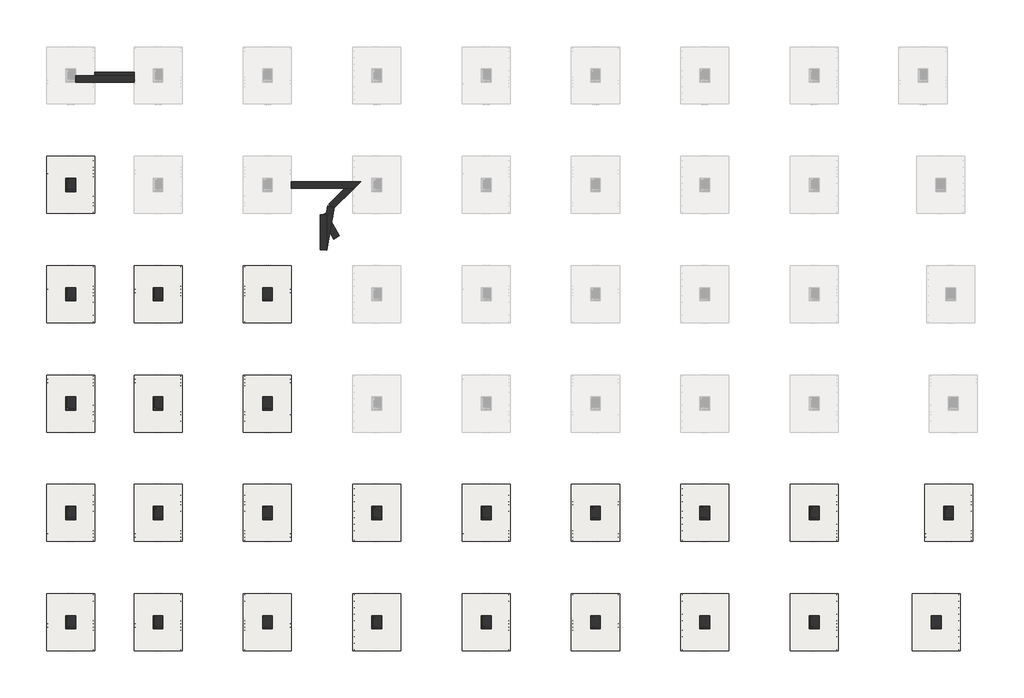
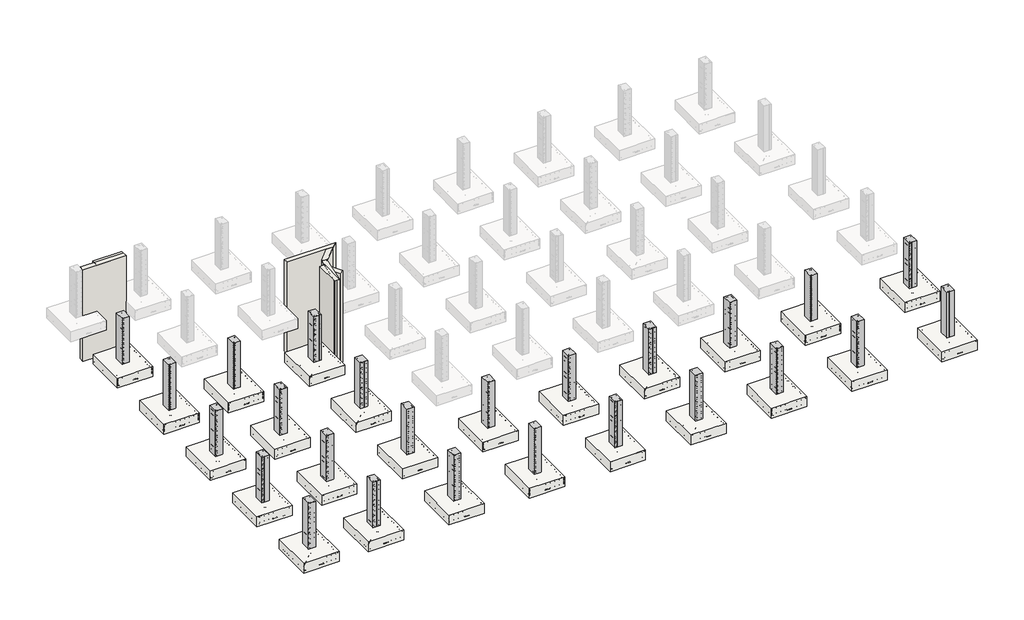
# One storey, part 1 of 33: 25 columns, 25 slabs, 9 walls.
"""IFC4 building model written with IfcOpenShell, lengths in millimetres."""

from ifc_helpers import new_model, si_unit, frame, origin, place, context, project, spatial, polyline, outline, extrude, faceted_brep, element, save

model = new_model("IFC4")

# Units and contexts
model_context = context("Model", 3, world=origin())
ifc_project = project(units=[si_unit("LENGTHUNIT", "METRE", prefix="MILLI")], contexts=[model_context])

# Site, building, storey
site = spatial("IfcSite", under=ifc_project)
building = spatial("IfcBuilding", under=site)
storey = spatial("IfcBuildingStorey", under=building, Elevation=-3000.0)

# Columns
placement = place(None, origin())
element("IfcColumn", 1, ObjectType="M_Concrete-Rectangular-Column : 300 x 450mm", at=placement, inside=storey, context=model_context, shape_type="SweptSolid", body=[
    extrude(outline(polyline([(-13414.8142742, 12007.0891866), (-13414.8142742, 11397.4891866), (-13864.8142742, 11397.4891866), (-13864.8142742, 12007.0891866), (-13414.8142742, 12007.0891866)])), frame((0.0, 0.0, -3000.0), z_axis=(0.0, 0.0, 1.0), x_axis=(1.0, 0.0, 0.0)), (0.0, 0.0, 1.0), 3000.0),
])
element("IfcColumn", 2, ObjectType="M_Concrete-Rectangular-Column : 300 x 450mm", at=placement, inside=storey, context=model_context, shape_type="SweptSolid", body=[
    extrude(outline(polyline([(-13414.8142742, 7007.0891866), (-13414.8142742, 6397.4891866), (-13864.8142742, 6397.4891866), (-13864.8142742, 7007.0891866), (-13414.8142742, 7007.0891866)])), frame((0.0, 0.0, -3000.0), z_axis=(0.0, 0.0, 1.0), x_axis=(1.0, 0.0, 0.0)), (0.0, 0.0, 1.0), 3000.0),
])
element("IfcColumn", 3, ObjectType="M_Concrete-Rectangular-Column : 300 x 450mm", at=placement, inside=storey, context=model_context, shape_type="SweptSolid", body=[
    extrude(outline(polyline([(-13414.8142742, 2007.0891866), (-13414.8142742, 1397.4891866), (-13864.8142742, 1397.4891866), (-13864.8142742, 2007.0891866), (-13414.8142742, 2007.0891866)])), frame((0.0, 0.0, -3000.0), z_axis=(0.0, 0.0, 1.0), x_axis=(1.0, 0.0, 0.0)), (0.0, 0.0, 1.0), 3000.0),
])
element("IfcColumn", 4, ObjectType="M_Concrete-Rectangular-Column : 300 x 450mm", at=placement, inside=storey, context=model_context, shape_type="SweptSolid", body=[
    extrude(outline(polyline([(-13414.8142742, -2992.9108134), (-13414.8142742, -3602.5108134), (-13864.8142742, -3602.5108134), (-13864.8142742, -2992.9108134), (-13414.8142742, -2992.9108134)])), frame((0.0, 0.0, -3000.0), z_axis=(0.0, 0.0, 1.0), x_axis=(1.0, 0.0, 0.0)), (0.0, 0.0, 1.0), 3000.0),
])
element("IfcColumn", 5, ObjectType="M_Concrete-Rectangular-Column : 300 x 450mm", at=placement, inside=storey, context=model_context, shape_type="SweptSolid", body=[
    extrude(outline(polyline([(-13414.8142742, -7992.9108134), (-13414.8142742, -8602.5108134), (-13864.8142742, -8602.5108134), (-13864.8142742, -7992.9108134), (-13414.8142742, -7992.9108134)])), frame((0.0, 0.0, -3000.0), z_axis=(0.0, 0.0, 1.0), x_axis=(1.0, 0.0, 0.0)), (0.0, 0.0, 1.0), 3000.0),
])
element("IfcColumn", 6, ObjectType="M_Concrete-Rectangular-Column : 300 x 450mm", at=placement, inside=storey, context=model_context, shape_type="SweptSolid", body=[
    extrude(outline(polyline([(-9414.8142742, 7007.0891866), (-9414.8142742, 6397.4891866), (-9864.8142742, 6397.4891866), (-9864.8142742, 7007.0891866), (-9414.8142742, 7007.0891866)])), frame((0.0, 0.0, -3000.0), z_axis=(0.0, 0.0, 1.0), x_axis=(1.0, 0.0, 0.0)), (0.0, 0.0, 1.0), 3000.0),
])
element("IfcColumn", 7, ObjectType="M_Concrete-Rectangular-Column : 300 x 450mm", at=placement, inside=storey, context=model_context, shape_type="SweptSolid", body=[
    extrude(outline(polyline([(-9414.8142742, 2007.0891866), (-9414.8142742, 1397.4891866), (-9864.8142742, 1397.4891866), (-9864.8142742, 2007.0891866), (-9414.8142742, 2007.0891866)])), frame((0.0, 0.0, -3000.0), z_axis=(0.0, 0.0, 1.0), x_axis=(1.0, 0.0, 0.0)), (0.0, 0.0, 1.0), 3000.0),
])
element("IfcColumn", 8, ObjectType="M_Concrete-Rectangular-Column : 300 x 450mm", at=placement, inside=storey, context=model_context, shape_type="SweptSolid", body=[
    extrude(outline(polyline([(-9414.8142742, -2992.9108134), (-9414.8142742, -3602.5108134), (-9864.8142742, -3602.5108134), (-9864.8142742, -2992.9108134), (-9414.8142742, -2992.9108134)])), frame((0.0, 0.0, -3000.0), z_axis=(0.0, 0.0, 1.0), x_axis=(1.0, 0.0, 0.0)), (0.0, 0.0, 1.0), 3000.0),
])
element("IfcColumn", 9, ObjectType="M_Concrete-Rectangular-Column : 300 x 450mm", at=placement, inside=storey, context=model_context, shape_type="SweptSolid", body=[
    extrude(outline(polyline([(-9414.8142742, -7992.9108134), (-9414.8142742, -8602.5108134), (-9864.8142742, -8602.5108134), (-9864.8142742, -7992.9108134), (-9414.8142742, -7992.9108134)])), frame((0.0, 0.0, -3000.0), z_axis=(0.0, 0.0, 1.0), x_axis=(1.0, 0.0, 0.0)), (0.0, 0.0, 1.0), 3000.0),
])
element("IfcColumn", 10, ObjectType="M_Concrete-Rectangular-Column : 300 x 450mm", at=placement, inside=storey, context=model_context, shape_type="SweptSolid", body=[
    extrude(outline(polyline([(-4414.8142742, 7007.0891866), (-4414.8142742, 6397.4891866), (-4864.8142742, 6397.4891866), (-4864.8142742, 7007.0891866), (-4414.8142742, 7007.0891866)])), frame((0.0, 0.0, -3000.0), z_axis=(0.0, 0.0, 1.0), x_axis=(1.0, 0.0, 0.0)), (0.0, 0.0, 1.0), 3000.0),
])
element("IfcColumn", 11, ObjectType="M_Concrete-Rectangular-Column : 300 x 450mm", at=placement, inside=storey, context=model_context, shape_type="SweptSolid", body=[
    extrude(outline(polyline([(-4414.8142742, 2007.0891866), (-4414.8142742, 1397.4891866), (-4864.8142742, 1397.4891866), (-4864.8142742, 2007.0891866), (-4414.8142742, 2007.0891866)])), frame((0.0, 0.0, -3000.0), z_axis=(0.0, 0.0, 1.0), x_axis=(1.0, 0.0, 0.0)), (0.0, 0.0, 1.0), 3000.0),
])
element("IfcColumn", 12, ObjectType="M_Concrete-Rectangular-Column : 300 x 450mm", at=placement, inside=storey, context=model_context, shape_type="SweptSolid", body=[
    extrude(outline(polyline([(-4414.8142742, -2992.9108134), (-4414.8142742, -3602.5108134), (-4864.8142742, -3602.5108134), (-4864.8142742, -2992.9108134), (-4414.8142742, -2992.9108134)])), frame((0.0, 0.0, -3000.0), z_axis=(0.0, 0.0, 1.0), x_axis=(1.0, 0.0, 0.0)), (0.0, 0.0, 1.0), 3000.0),
])
element("IfcColumn", 13, ObjectType="M_Concrete-Rectangular-Column : 300 x 450mm", at=placement, inside=storey, context=model_context, shape_type="SweptSolid", body=[
    extrude(outline(polyline([(-4414.8142742, -7992.9108134), (-4414.8142742, -8602.5108134), (-4864.8142742, -8602.5108134), (-4864.8142742, -7992.9108134), (-4414.8142742, -7992.9108134)])), frame((0.0, 0.0, -3000.0), z_axis=(0.0, 0.0, 1.0), x_axis=(1.0, 0.0, 0.0)), (0.0, 0.0, 1.0), 3000.0),
])
element("IfcColumn", 14, ObjectType="M_Concrete-Rectangular-Column : 300 x 450mm", at=placement, inside=storey, context=model_context, shape_type="SweptSolid", body=[
    extrude(outline(polyline([(585.1857258, -2992.9108134), (585.1857258, -3602.5108134), (135.1857258, -3602.5108134), (135.1857258, -2992.9108134), (585.1857258, -2992.9108134)])), frame((0.0, 0.0, -3000.0), z_axis=(0.0, 0.0, 1.0), x_axis=(1.0, 0.0, 0.0)), (0.0, 0.0, 1.0), 3000.0),
])
element("IfcColumn", 15, ObjectType="M_Concrete-Rectangular-Column : 300 x 450mm", at=placement, inside=storey, context=model_context, shape_type="SweptSolid", body=[
    extrude(outline(polyline([(585.1857258, -7992.9108134), (585.1857258, -8602.5108134), (135.1857258, -8602.5108134), (135.1857258, -7992.9108134), (585.1857258, -7992.9108134)])), frame((0.0, 0.0, -3000.0), z_axis=(0.0, 0.0, 1.0), x_axis=(1.0, 0.0, 0.0)), (0.0, 0.0, 1.0), 3000.0),
])
element("IfcColumn", 16, ObjectType="M_Concrete-Rectangular-Column : 300 x 450mm", at=placement, inside=storey, context=model_context, shape_type="SweptSolid", body=[
    extrude(outline(polyline([(5585.1857258, -2992.9108134), (5585.1857258, -3602.5108134), (5135.1857258, -3602.5108134), (5135.1857258, -2992.9108134), (5585.1857258, -2992.9108134)])), frame((0.0, 0.0, -3000.0), z_axis=(0.0, 0.0, 1.0), x_axis=(1.0, 0.0, 0.0)), (0.0, 0.0, 1.0), 3000.0),
])
element("IfcColumn", 17, ObjectType="M_Concrete-Rectangular-Column : 300 x 450mm", at=placement, inside=storey, context=model_context, shape_type="SweptSolid", body=[
    extrude(outline(polyline([(5585.1857258, -7992.9108134), (5585.1857258, -8602.5108134), (5135.1857258, -8602.5108134), (5135.1857258, -7992.9108134), (5585.1857258, -7992.9108134)])), frame((0.0, 0.0, -3000.0), z_axis=(0.0, 0.0, 1.0), x_axis=(1.0, 0.0, 0.0)), (0.0, 0.0, 1.0), 3000.0),
])
element("IfcColumn", 18, ObjectType="M_Concrete-Rectangular-Column : 300 x 450mm", at=placement, inside=storey, context=model_context, shape_type="SweptSolid", body=[
    extrude(outline(polyline([(10585.1857258, -2992.9108134), (10585.1857258, -3602.5108134), (10135.1857258, -3602.5108134), (10135.1857258, -2992.9108134), (10585.1857258, -2992.9108134)])), frame((0.0, 0.0, -3000.0), z_axis=(0.0, 0.0, 1.0), x_axis=(1.0, 0.0, 0.0)), (0.0, 0.0, 1.0), 3000.0),
])
element("IfcColumn", 19, ObjectType="M_Concrete-Rectangular-Column : 300 x 450mm", at=placement, inside=storey, context=model_context, shape_type="SweptSolid", body=[
    extrude(outline(polyline([(10585.1857258, -7992.9108134), (10585.1857258, -8602.5108134), (10135.1857258, -8602.5108134), (10135.1857258, -7992.9108134), (10585.1857258, -7992.9108134)])), frame((0.0, 0.0, -3000.0), z_axis=(0.0, 0.0, 1.0), x_axis=(1.0, 0.0, 0.0)), (0.0, 0.0, 1.0), 3000.0),
])
element("IfcColumn", 20, ObjectType="M_Concrete-Rectangular-Column : 300 x 450mm", at=placement, inside=storey, context=model_context, shape_type="SweptSolid", body=[
    extrude(outline(polyline([(15585.1857258, -2992.9108134), (15585.1857258, -3602.5108134), (15135.1857258, -3602.5108134), (15135.1857258, -2992.9108134), (15585.1857258, -2992.9108134)])), frame((0.0, 0.0, -3000.0), z_axis=(0.0, 0.0, 1.0), x_axis=(1.0, 0.0, 0.0)), (0.0, 0.0, 1.0), 3000.0),
])
element("IfcColumn", 21, ObjectType="M_Concrete-Rectangular-Column : 300 x 450mm", at=placement, inside=storey, context=model_context, shape_type="SweptSolid", body=[
    extrude(outline(polyline([(15585.1857258, -7992.9108134), (15585.1857258, -8602.5108134), (15135.1857258, -8602.5108134), (15135.1857258, -7992.9108134), (15585.1857258, -7992.9108134)])), frame((0.0, 0.0, -3000.0), z_axis=(0.0, 0.0, 1.0), x_axis=(1.0, 0.0, 0.0)), (0.0, 0.0, 1.0), 3000.0),
])
element("IfcColumn", 22, ObjectType="M_Concrete-Rectangular-Column : 300 x 450mm", at=placement, inside=storey, context=model_context, shape_type="SweptSolid", body=[
    extrude(outline(polyline([(20585.1857258, -2992.9108134), (20585.1857258, -3602.5108134), (20135.1857258, -3602.5108134), (20135.1857258, -2992.9108134), (20585.1857258, -2992.9108134)])), frame((0.0, 0.0, -3000.0), z_axis=(0.0, 0.0, 1.0), x_axis=(1.0, 0.0, 0.0)), (0.0, 0.0, 1.0), 3000.0),
])
element("IfcColumn", 23, ObjectType="M_Concrete-Rectangular-Column : 300 x 450mm", at=placement, inside=storey, context=model_context, shape_type="SweptSolid", body=[
    extrude(outline(polyline([(20585.1857258, -7992.9108134), (20585.1857258, -8602.5108134), (20135.1857258, -8602.5108134), (20135.1857258, -7992.9108134), (20585.1857258, -7992.9108134)])), frame((0.0, 0.0, -3000.0), z_axis=(0.0, 0.0, 1.0), x_axis=(1.0, 0.0, 0.0)), (0.0, 0.0, 1.0), 3000.0),
])
element("IfcColumn", 24, ObjectType="M_Concrete-Rectangular-Column : 300 x 450mm", at=placement, inside=storey, context=model_context, shape_type="SweptSolid", body=[
    extrude(outline(polyline([(26731.4237106, -2992.9108134), (26731.4237106, -3602.5108134), (26281.4237106, -3602.5108134), (26281.4237106, -2992.9108134), (26731.4237106, -2992.9108134)])), frame((0.0, 0.0, -3000.0), z_axis=(0.0, 0.0, 1.0), x_axis=(1.0, 0.0, 0.0)), (0.0, 0.0, 1.0), 3000.0),
])
element("IfcColumn", 25, ObjectType="M_Concrete-Rectangular-Column : 300 x 450mm", at=placement, inside=storey, context=model_context, shape_type="SweptSolid", body=[
    extrude(outline(polyline([(26167.6833949, -7992.9108134), (26167.6833949, -8602.5108134), (25717.6833949, -8602.5108134), (25717.6833949, -7992.9108134), (26167.6833949, -7992.9108134)])), frame((0.0, 0.0, -3000.0), z_axis=(0.0, 0.0, 1.0), x_axis=(1.0, 0.0, 0.0)), (0.0, 0.0, 1.0), 3000.0),
])

# Slabs
element("IfcSlab", 26, ObjectType="M_Footing-Rectangular : 650X2200X2600", at=placement, inside=storey, context=model_context, shape_type="SweptSolid", body=[
    extrude(outline(polyline([(-12539.8142742, 13002.2891866), (-12539.8142742, 10402.2891866), (-14739.8142742, 10402.2891866), (-14739.8142742, 13002.2891866), (-12539.8142742, 13002.2891866)])), frame((0.0, 0.0, -3650.0), z_axis=(0.0, 0.0, 1.0), x_axis=(1.0, 0.0, 0.0)), (0.0, 0.0, 1.0), 650.0),
])
element("IfcSlab", 27, ObjectType="M_Footing-Rectangular : 650X2200X2600", at=placement, inside=storey, context=model_context, shape_type="SweptSolid", body=[
    extrude(outline(polyline([(-12539.8142742, 8002.2891866), (-12539.8142742, 5402.2891866), (-14739.8142742, 5402.2891866), (-14739.8142742, 8002.2891866), (-12539.8142742, 8002.2891866)])), frame((0.0, 0.0, -3650.0), z_axis=(0.0, 0.0, 1.0), x_axis=(1.0, 0.0, 0.0)), (0.0, 0.0, 1.0), 650.0),
])
element("IfcSlab", 28, ObjectType="M_Footing-Rectangular : 650X2200X2600", at=placement, inside=storey, context=model_context, shape_type="SweptSolid", body=[
    extrude(outline(polyline([(-12539.8142742, 3002.2891866), (-12539.8142742, 402.2891866), (-14739.8142742, 402.2891866), (-14739.8142742, 3002.2891866), (-12539.8142742, 3002.2891866)])), frame((0.0, 0.0, -3650.0), z_axis=(0.0, 0.0, 1.0), x_axis=(1.0, 0.0, 0.0)), (0.0, 0.0, 1.0), 650.0),
])
element("IfcSlab", 29, ObjectType="M_Footing-Rectangular : 650X2200X2600", at=placement, inside=storey, context=model_context, shape_type="SweptSolid", body=[
    extrude(outline(polyline([(-12539.8142742, -1997.7108134), (-12539.8142742, -4597.7108134), (-14739.8142742, -4597.7108134), (-14739.8142742, -1997.7108134), (-12539.8142742, -1997.7108134)])), frame((0.0, 0.0, -3650.0), z_axis=(0.0, 0.0, 1.0), x_axis=(1.0, 0.0, 0.0)), (0.0, 0.0, 1.0), 650.0),
])
element("IfcSlab", 30, ObjectType="M_Footing-Rectangular : 650X2200X2600", at=placement, inside=storey, context=model_context, shape_type="SweptSolid", body=[
    extrude(outline(polyline([(-12539.8142742, -6997.7108134), (-12539.8142742, -9597.7108134), (-14739.8142742, -9597.7108134), (-14739.8142742, -6997.7108134), (-12539.8142742, -6997.7108134)])), frame((0.0, 0.0, -3650.0), z_axis=(0.0, 0.0, 1.0), x_axis=(1.0, 0.0, 0.0)), (0.0, 0.0, 1.0), 650.0),
])
element("IfcSlab", 31, ObjectType="M_Footing-Rectangular : 650X2200X2600", at=placement, inside=storey, context=model_context, shape_type="SweptSolid", body=[
    extrude(outline(polyline([(-8539.8142742, 8002.2891866), (-8539.8142742, 5402.2891866), (-10739.8142742, 5402.2891866), (-10739.8142742, 8002.2891866), (-8539.8142742, 8002.2891866)])), frame((0.0, 0.0, -3650.0), z_axis=(0.0, 0.0, 1.0), x_axis=(1.0, 0.0, 0.0)), (0.0, 0.0, 1.0), 650.0),
])
element("IfcSlab", 32, ObjectType="M_Footing-Rectangular : 650X2200X2600", at=placement, inside=storey, context=model_context, shape_type="SweptSolid", body=[
    extrude(outline(polyline([(-8539.8142742, 3002.2891866), (-8539.8142742, 402.2891866), (-10739.8142742, 402.2891866), (-10739.8142742, 3002.2891866), (-8539.8142742, 3002.2891866)])), frame((0.0, 0.0, -3650.0), z_axis=(0.0, 0.0, 1.0), x_axis=(1.0, 0.0, 0.0)), (0.0, 0.0, 1.0), 650.0),
])
element("IfcSlab", 33, ObjectType="M_Footing-Rectangular : 650X2200X2600", at=placement, inside=storey, context=model_context, shape_type="SweptSolid", body=[
    extrude(outline(polyline([(-8539.8142742, -1997.7108134), (-8539.8142742, -4597.7108134), (-10739.8142742, -4597.7108134), (-10739.8142742, -1997.7108134), (-8539.8142742, -1997.7108134)])), frame((0.0, 0.0, -3650.0), z_axis=(0.0, 0.0, 1.0), x_axis=(1.0, 0.0, 0.0)), (0.0, 0.0, 1.0), 650.0),
])
element("IfcSlab", 34, ObjectType="M_Footing-Rectangular : 650X2200X2600", at=placement, inside=storey, context=model_context, shape_type="SweptSolid", body=[
    extrude(outline(polyline([(-8539.8142742, -6997.7108134), (-8539.8142742, -9597.7108134), (-10739.8142742, -9597.7108134), (-10739.8142742, -6997.7108134), (-8539.8142742, -6997.7108134)])), frame((0.0, 0.0, -3650.0), z_axis=(0.0, 0.0, 1.0), x_axis=(1.0, 0.0, 0.0)), (0.0, 0.0, 1.0), 650.0),
])
element("IfcSlab", 35, ObjectType="M_Footing-Rectangular : 650X2200X2600", at=placement, inside=storey, context=model_context, shape_type="SweptSolid", body=[
    extrude(outline(polyline([(-3539.8142742, 8002.2891866), (-3539.8142742, 5402.2891866), (-5739.8142742, 5402.2891866), (-5739.8142742, 8002.2891866), (-3539.8142742, 8002.2891866)])), frame((0.0, 0.0, -3650.0), z_axis=(0.0, 0.0, 1.0), x_axis=(1.0, 0.0, 0.0)), (0.0, 0.0, 1.0), 650.0),
])
element("IfcSlab", 36, ObjectType="M_Footing-Rectangular : 650X2200X2600", at=placement, inside=storey, context=model_context, shape_type="SweptSolid", body=[
    extrude(outline(polyline([(-3539.8142742, 3002.2891866), (-3539.8142742, 402.2891866), (-5739.8142742, 402.2891866), (-5739.8142742, 3002.2891866), (-3539.8142742, 3002.2891866)])), frame((0.0, 0.0, -3650.0), z_axis=(0.0, 0.0, 1.0), x_axis=(1.0, 0.0, 0.0)), (0.0, 0.0, 1.0), 650.0),
])
element("IfcSlab", 37, ObjectType="M_Footing-Rectangular : 650X2200X2600", at=placement, inside=storey, context=model_context, shape_type="SweptSolid", body=[
    extrude(outline(polyline([(-3539.8142742, -1997.7108134), (-3539.8142742, -4597.7108134), (-5739.8142742, -4597.7108134), (-5739.8142742, -1997.7108134), (-3539.8142742, -1997.7108134)])), frame((0.0, 0.0, -3650.0), z_axis=(0.0, 0.0, 1.0), x_axis=(1.0, 0.0, 0.0)), (0.0, 0.0, 1.0), 650.0),
])
element("IfcSlab", 38, ObjectType="M_Footing-Rectangular : 650X2200X2600", at=placement, inside=storey, context=model_context, shape_type="SweptSolid", body=[
    extrude(outline(polyline([(-3539.8142742, -6997.7108134), (-3539.8142742, -9597.7108134), (-5739.8142742, -9597.7108134), (-5739.8142742, -6997.7108134), (-3539.8142742, -6997.7108134)])), frame((0.0, 0.0, -3650.0), z_axis=(0.0, 0.0, 1.0), x_axis=(1.0, 0.0, 0.0)), (0.0, 0.0, 1.0), 650.0),
])
element("IfcSlab", 39, ObjectType="M_Footing-Rectangular : 650X2200X2600", at=placement, inside=storey, context=model_context, shape_type="SweptSolid", body=[
    extrude(outline(polyline([(1460.1857258, -1997.7108134), (1460.1857258, -4597.7108134), (-739.8142742, -4597.7108134), (-739.8142742, -1997.7108134), (1460.1857258, -1997.7108134)])), frame((0.0, 0.0, -3650.0), z_axis=(0.0, 0.0, 1.0), x_axis=(1.0, 0.0, 0.0)), (0.0, 0.0, 1.0), 650.0),
])
element("IfcSlab", 40, ObjectType="M_Footing-Rectangular : 650X2200X2600", at=placement, inside=storey, context=model_context, shape_type="SweptSolid", body=[
    extrude(outline(polyline([(1460.1857258, -6997.7108134), (1460.1857258, -9597.7108134), (-739.8142742, -9597.7108134), (-739.8142742, -6997.7108134), (1460.1857258, -6997.7108134)])), frame((0.0, 0.0, -3650.0), z_axis=(0.0, 0.0, 1.0), x_axis=(1.0, 0.0, 0.0)), (0.0, 0.0, 1.0), 650.0),
])
element("IfcSlab", 41, ObjectType="M_Footing-Rectangular : 650X2200X2600", at=placement, inside=storey, context=model_context, shape_type="SweptSolid", body=[
    extrude(outline(polyline([(6460.1857258, -1997.7108134), (6460.1857258, -4597.7108134), (4260.1857258, -4597.7108134), (4260.1857258, -1997.7108134), (6460.1857258, -1997.7108134)])), frame((0.0, 0.0, -3650.0), z_axis=(0.0, 0.0, 1.0), x_axis=(1.0, 0.0, 0.0)), (0.0, 0.0, 1.0), 650.0),
])
element("IfcSlab", 42, ObjectType="M_Footing-Rectangular : 650X2200X2600", at=placement, inside=storey, context=model_context, shape_type="SweptSolid", body=[
    extrude(outline(polyline([(6460.1857258, -6997.7108134), (6460.1857258, -9597.7108134), (4260.1857258, -9597.7108134), (4260.1857258, -6997.7108134), (6460.1857258, -6997.7108134)])), frame((0.0, 0.0, -3650.0), z_axis=(0.0, 0.0, 1.0), x_axis=(1.0, 0.0, 0.0)), (0.0, 0.0, 1.0), 650.0),
])
element("IfcSlab", 43, ObjectType="M_Footing-Rectangular : 650X2200X2600", at=placement, inside=storey, context=model_context, shape_type="SweptSolid", body=[
    extrude(outline(polyline([(11460.1857258, -1997.7108134), (11460.1857258, -4597.7108134), (9260.1857258, -4597.7108134), (9260.1857258, -1997.7108134), (11460.1857258, -1997.7108134)])), frame((0.0, 0.0, -3650.0), z_axis=(0.0, 0.0, 1.0), x_axis=(1.0, 0.0, 0.0)), (0.0, 0.0, 1.0), 650.0),
])
element("IfcSlab", 44, ObjectType="M_Footing-Rectangular : 650X2200X2600", at=placement, inside=storey, context=model_context, shape_type="SweptSolid", body=[
    extrude(outline(polyline([(11460.1857258, -6997.7108134), (11460.1857258, -9597.7108134), (9260.1857258, -9597.7108134), (9260.1857258, -6997.7108134), (11460.1857258, -6997.7108134)])), frame((0.0, 0.0, -3650.0), z_axis=(0.0, 0.0, 1.0), x_axis=(1.0, 0.0, 0.0)), (0.0, 0.0, 1.0), 650.0),
])
element("IfcSlab", 45, ObjectType="M_Footing-Rectangular : 650X2200X2600", at=placement, inside=storey, context=model_context, shape_type="SweptSolid", body=[
    extrude(outline(polyline([(16460.1857258, -1997.7108134), (16460.1857258, -4597.7108134), (14260.1857258, -4597.7108134), (14260.1857258, -1997.7108134), (16460.1857258, -1997.7108134)])), frame((0.0, 0.0, -3650.0), z_axis=(0.0, 0.0, 1.0), x_axis=(1.0, 0.0, 0.0)), (0.0, 0.0, 1.0), 650.0),
])
element("IfcSlab", 46, ObjectType="M_Footing-Rectangular : 650X2200X2600", at=placement, inside=storey, context=model_context, shape_type="SweptSolid", body=[
    extrude(outline(polyline([(16460.1857258, -6997.7108134), (16460.1857258, -9597.7108134), (14260.1857258, -9597.7108134), (14260.1857258, -6997.7108134), (16460.1857258, -6997.7108134)])), frame((0.0, 0.0, -3650.0), z_axis=(0.0, 0.0, 1.0), x_axis=(1.0, 0.0, 0.0)), (0.0, 0.0, 1.0), 650.0),
])
element("IfcSlab", 47, ObjectType="M_Footing-Rectangular : 650X2200X2600", at=placement, inside=storey, context=model_context, shape_type="SweptSolid", body=[
    extrude(outline(polyline([(21460.1857258, -1997.7108134), (21460.1857258, -4597.7108134), (19260.1857258, -4597.7108134), (19260.1857258, -1997.7108134), (21460.1857258, -1997.7108134)])), frame((0.0, 0.0, -3650.0), z_axis=(0.0, 0.0, 1.0), x_axis=(1.0, 0.0, 0.0)), (0.0, 0.0, 1.0), 650.0),
])
element("IfcSlab", 48, ObjectType="M_Footing-Rectangular : 650X2200X2600", at=placement, inside=storey, context=model_context, shape_type="SweptSolid", body=[
    extrude(outline(polyline([(21460.1857258, -6997.7108134), (21460.1857258, -9597.7108134), (19260.1857258, -9597.7108134), (19260.1857258, -6997.7108134), (21460.1857258, -6997.7108134)])), frame((0.0, 0.0, -3650.0), z_axis=(0.0, 0.0, 1.0), x_axis=(1.0, 0.0, 0.0)), (0.0, 0.0, 1.0), 650.0),
])
element("IfcSlab", 49, ObjectType="M_Footing-Rectangular : 650X2200X2600", at=placement, inside=storey, context=model_context, shape_type="SweptSolid", body=[
    extrude(outline(polyline([(27606.4237106, -1997.7108134), (27606.4237106, -4597.7108134), (25406.4237106, -4597.7108134), (25406.4237106, -1997.7108134), (27606.4237106, -1997.7108134)])), frame((0.0, 0.0, -3650.0), z_axis=(0.0, 0.0, 1.0), x_axis=(1.0, 0.0, 0.0)), (0.0, 0.0, 1.0), 650.0),
])
element("IfcSlab", 50, ObjectType="M_Footing-Rectangular : 650X2200X2600", at=placement, inside=storey, context=model_context, shape_type="SweptSolid", body=[
    extrude(outline(polyline([(27042.6833949, -6997.7108134), (27042.6833949, -9597.7108134), (24842.6833949, -9597.7108134), (24842.6833949, -6997.7108134), (27042.6833949, -6997.7108134)])), frame((0.0, 0.0, -3650.0), z_axis=(0.0, 0.0, 1.0), x_axis=(1.0, 0.0, 0.0)), (0.0, 0.0, 1.0), 650.0),
])

# Walls
element("IfcWall", 51, ObjectType="wall", at=placement, inside=storey, context=model_context, shape_type="SweptSolid", body=[
    extrude(outline(polyline([(-10739.8142742, 16549.7891866), (-12539.8142742, 16549.7891866), (-12539.8142742, 16854.7891866), (-10739.8142742, 16854.7891866), (-10739.8142742, 16549.7891866)])), frame((0.0, 0.0, -6000.0), z_axis=(0.0, 0.0, 1.0), x_axis=(1.0, 0.0, 0.0)), (0.0, 0.0, 1.0), 6000.0),
])
element("IfcWall", 52, ObjectType="wall", at=placement, inside=storey, context=model_context, shape_type="SweptSolid", body=[
    extrude(outline(polyline([(-10739.8142742, 16549.7891866), (-12539.8142742, 16549.7891866), (-12539.8142742, 16854.7891866), (-10739.8142742, 16854.7891866), (-10739.8142742, 16549.7891866)])), frame((0.0, 0.0, -6000.0), z_axis=(0.0, 0.0, 1.0), x_axis=(1.0, 0.0, 0.0)), (0.0, 0.0, 1.0), 6000.0),
])
element("IfcWall", 53, ObjectType="wall", at=placement, inside=storey, context=model_context, shape_type="Brep", body=[
    faceted_brep([(-3539.8142742, 11549.7891866, -6000.0), (-1107.9818425, 11549.7891866, -6000.0), (-676.646706, 11549.7891866, -6000.0), (-676.646706, 11549.7891866, 0.0), (-1107.9818425, 11549.7891866, 0.0), (-3539.8142742, 11549.7891866, 0.0), (-3539.8142742, 11854.7891866, -6000.0), (-3539.8142742, 11854.7891866, 0.0), (-371.646706, 11854.7891866, 0.0), (-371.646706, 11854.7891866, -6000.0)], [[[0, 1, 2, 3, 4, 5]], [[6, 7, 8, 9]], [[2, 1, 0, 6, 9]], [[5, 4, 3, 8, 7]], [[0, 5, 7, 6]], [[3, 2, 9, 8]]]),
])
element("IfcWall", 54, ObjectType="wall", at=placement, inside=storey, context=model_context, shape_type="SweptSolid", body=[
    extrude(outline(polyline([(-1837.597552, 10820.1734771), (-1107.9818425, 11549.7891866), (-676.646706, 11549.7891866), (-1621.9299837, 10604.5059088), (-1837.597552, 10820.1734771)])), frame((0.0, 0.0, -6000.0), z_axis=(0.0, 0.0, 1.0), x_axis=(1.0, 0.0, 0.0)), (0.0, 0.0, 1.0), 6000.0),
])
element("IfcWall", 55, ObjectType="wall", at=placement, inside=storey, context=model_context, shape_type="SweptSolid", body=[
    extrude(outline(polyline([(-2227.2433055, 8769.205534), (-1879.9469502, 10738.8210401), (-1579.5805855, 10685.8583459), (-1926.8769409, 8716.2428399), (-2227.2433055, 8769.205534)])), frame((0.0, 0.0, -6000.0), z_axis=(0.0, 0.0, 1.0), x_axis=(1.0, 0.0, 0.0)), (0.0, 0.0, 1.0), 6000.0),
])
element("IfcWall", 56, ObjectType="wall", at=placement, inside=storey, context=model_context, shape_type="SweptSolid", body=[
    extrude(outline(polyline([(-1924.5601232, 10342.724187), (-1924.5601232, 8742.724187), (-2229.5601232, 8742.724187), (-2229.5601232, 10342.724187), (-1924.5601232, 10342.724187)])), frame((0.0, 0.0, -6000.0), z_axis=(0.0, 0.0, 1.0), x_axis=(1.0, 0.0, 0.0)), (0.0, 0.0, 1.0), 6000.0),
])
element("IfcWall", 57, ObjectType="wall", at=placement, inside=storey, context=model_context, shape_type="SweptSolid", body=[
    extrude(outline(polyline([(-1609.1289973, 9227.2437024), (-2209.1289973, 10266.474187), (-1944.9912491, 10418.974187), (-1344.9912491, 9379.7437024), (-1609.1289973, 9227.2437024)])), frame((0.0, 0.0, -6000.0), z_axis=(0.0, 0.0, 1.0), x_axis=(1.0, 0.0, 0.0)), (0.0, 0.0, 1.0), 6000.0),
])
element("IfcWall", 58, ObjectType="wall", at=placement, inside=storey, context=model_context, shape_type="SweptSolid", body=[
    extrude(outline(polyline([(-10739.8142742, 16397.2891866), (-12539.8142742, 16397.2891866), (-12539.8142742, 16702.2891866), (-10739.8142742, 16702.2891866), (-10739.8142742, 16397.2891866)])), frame((0.0, 0.0, -6000.0), z_axis=(0.0, 0.0, 1.0), x_axis=(1.0, 0.0, 0.0)), (0.0, 0.0, 1.0), 6000.0),
])
element("IfcWall", 59, ObjectType="wall", at=placement, inside=storey, context=model_context, shape_type="SweptSolid", body=[
    extrude(outline(polyline([(-10739.8142742, 16397.2891866), (-13414.8142742, 16397.2891866), (-13414.8142742, 16702.2891866), (-10739.8142742, 16702.2891866), (-10739.8142742, 16397.2891866)])), frame((0.0, 0.0, -6000.0), z_axis=(0.0, 0.0, 1.0), x_axis=(1.0, 0.0, 0.0)), (0.0, 0.0, 1.0), 6000.0),
])

save(model, "model.ifc")

# Revit data of these elements
# Grids (mm)
#   "D": line (31931.04, 1702.289) -> (-21764.969, 1702.289)
#   "F": line (31931.04, -8297.711) -> (-21764.969, -8297.711)
#   "E": line (31931.04, -3297.711) -> (-21764.969, -3297.711)
#   "15": arc centre (-46938.144, 2451.242) radius 73669.227 angles 6.052516 to 6.513854 rad from (1, 0)
#   "1": line (-13639.814, 19294.166) -> (-13639.814, -16890.777)
#   "2": line (-9639.814, 19294.166) -> (-9639.814, -16890.777)
#   "3": line (-4639.814, 19294.166) -> (-4639.814, -16890.777)
#   "4": line (360.186, 19294.166) -> (360.186, -16890.777)
#   "5": line (5360.186, 19294.166) -> (5360.186, -16890.777)
#   "6": line (10360.186, 19294.166) -> (10360.186, -16890.777)
#   "7": line (15360.186, 19294.166) -> (15360.186, -16890.777)
#   "8": line (20360.186, 19294.166) -> (20360.186, -16890.777)
#   "A": line (31931.04, 16702.289) -> (-21764.969, 16702.289)
#   "B": line (31931.04, 11702.289) -> (-21764.969, 11702.289)
#   "C": line (31931.04, 6702.289) -> (-21764.969, 6702.289)
# Type "M_Concrete-Rectangular-Column : 300 x 450mm"
#   b = 450 mm
#   h = 609.6 mm
#   Structural Material [instance default] = Concrete, Cast-in-Place gray
# Type "M_Footing-Rectangular : 650X2200X2600"
#   Width = 2200 mm
#   Length = 2600 mm
#   Foundation Thickness = 650 mm
#   Structural Material [instance default] = Concrete, Cast-in-Place gray
#   Assembly Code = ""
# Type "wall"
#   Layers, outside or top first: 305 mm no material (function 1)
# Elements 1, 2, 3, 4, 5, 6, 7, 8, 9, 10, 11, 12, 13, 14, 15, 16, 17, 18, 19, 20, 21, 22, 23, 24, 25 (IfcColumn, "M_Concrete-Rectangular-Column : 300 x 450mm")
#   Structural Material = Default New Material
#   Phase Created = New Construction
#   Materials on its faces: "Default New Material"
# Elements 26, 27, 28, 29, 30, 31, 32, 33, 34, 35, 36, 37, 38, 39, 40, 41, 42, 43, 44, 45, 46, 47, 48, 49, 50 (IfcSlab, "M_Footing-Rectangular : 650X2200X2600")
#   Structural Material = Concrete, Cast-in-Place gray
#   Phase Created = New Construction
#   Materials on its faces: "Concrete, Cast-in-Place gray"
# Elements 51, 52, 53, 54, 55, 56, 57, 58, 59 (IfcWall, "wall")
#   built-in parameter 1001111 = -3000 mm
#   Top Offset = 0 mm
#   Base Offset = -3000 mm
#   wall height = 6000 mm
#   Phase Created = New Construction
#   Materials on its faces: "Default Wall"
# Materials
#   "Concrete, Cast-in-Place gray": class "Concrete", colour RGB 130 132 119, transparency 0, Description = "Cast-in-place concrete", Cost = 0
#   "Default New Material": class "Generic", colour RGB 184 184 178, transparency 0, Cost = 0
#   "Default Wall": colour RGB 128 128 128, transparency 0, Cost = 0
